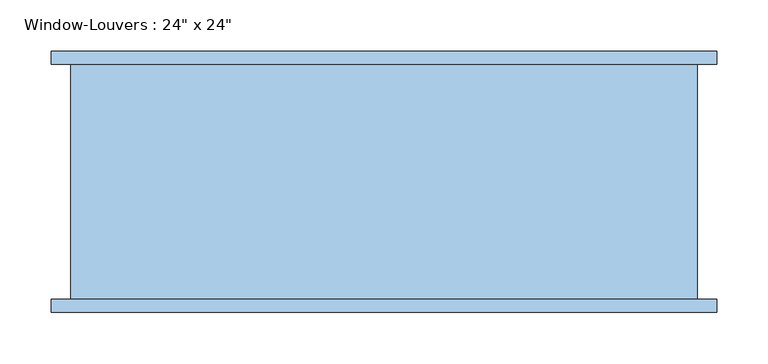
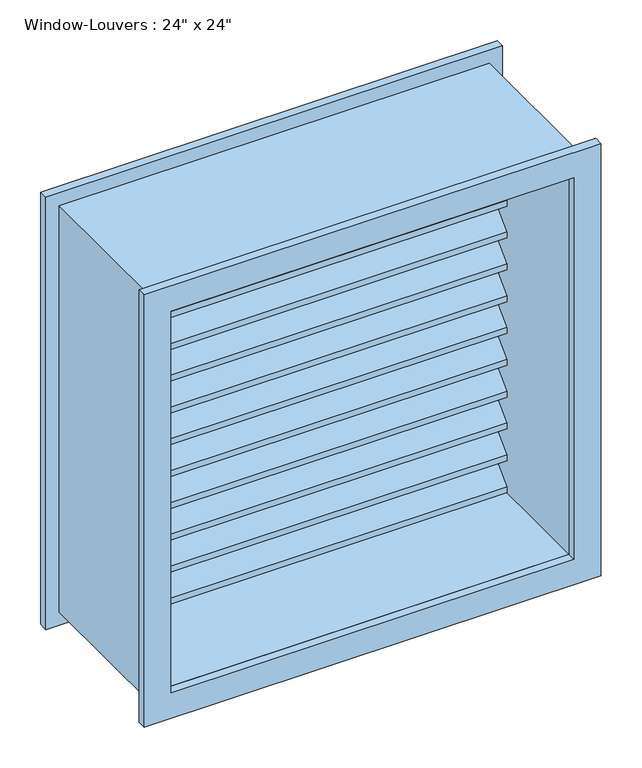
"""IFC4 building model written with IfcOpenShell, lengths in millimetres: window geometry."""

from ifc_helpers import new_model, si_unit, frame, origin, place, context, project, spatial, polyline, outline, extrude, source, transform, mapped, element, save


def window_f2d8fef0(model_context):
    return source(origin(), model_context, "Body", "SweptSolid", [
        extrude(outline(polyline([(107.95, 1419.1754778), (107.95, 1410.1952217), (69.85, 1448.2952217), (31.75, 1410.1952217), (31.75, 1419.1754778), (69.85, 1457.2754778), (107.95, 1419.1754778)])), frame((-285.75, 0.0, 0.0), z_axis=(1.0, 0.0, 0.0), x_axis=(0.0, 1.0, 0.0)), (0.0, 0.0, 1.0), 571.5),
        extrude(outline(polyline([(107.95, 1371.5009557), (107.95, 1362.5206995), (69.85, 1400.6206995), (31.75, 1362.5206995), (31.75, 1371.5009557), (69.85, 1409.6009557), (107.95, 1371.5009557)])), frame((-285.75, 0.0, 0.0), z_axis=(1.0, 0.0, 0.0), x_axis=(0.0, 1.0, 0.0)), (0.0, 0.0, 1.0), 571.5),
        extrude(outline(polyline([(107.95, 1323.8264335), (107.95, 1314.8461774), (69.85, 1352.9461774), (31.75, 1314.8461774), (31.75, 1323.8264335), (69.85, 1361.9264335), (107.95, 1323.8264335)])), frame((-285.75, 0.0, 0.0), z_axis=(1.0, 0.0, 0.0), x_axis=(0.0, 1.0, 0.0)), (0.0, 0.0, 1.0), 571.5),
        extrude(outline(polyline([(107.95, 1276.1519113), (107.95, 1267.1716552), (69.85, 1305.2716552), (31.75, 1267.1716552), (31.75, 1276.1519113), (69.85, 1314.2519113), (107.95, 1276.1519113)])), frame((-285.75, 0.0, 0.0), z_axis=(1.0, 0.0, 0.0), x_axis=(0.0, 1.0, 0.0)), (0.0, 0.0, 1.0), 571.5),
        extrude(outline(polyline([(107.95, 1228.4773891), (107.95, 1219.497133), (69.85, 1257.597133), (31.75, 1219.497133), (31.75, 1228.4773891), (69.85, 1266.5773891), (107.95, 1228.4773891)])), frame((-285.75, 0.0, 0.0), z_axis=(1.0, 0.0, 0.0), x_axis=(0.0, 1.0, 0.0)), (0.0, 0.0, 1.0), 571.5),
        extrude(outline(polyline([(107.95, 1180.802867), (107.95, 1171.8226109), (69.85, 1209.9226109), (31.75, 1171.8226109), (31.75, 1180.802867), (69.85, 1218.902867), (107.95, 1180.802867)])), frame((-285.75, 0.0, 0.0), z_axis=(1.0, 0.0, 0.0), x_axis=(0.0, 1.0, 0.0)), (0.0, 0.0, 1.0), 571.5),
        extrude(outline(polyline([(107.95, 1133.1283448), (107.95, 1124.1480887), (69.85, 1162.2480887), (31.75, 1124.1480887), (31.75, 1133.1283448), (69.85, 1171.2283448), (107.95, 1133.1283448)])), frame((-285.75, 0.0, 0.0), z_axis=(1.0, 0.0, 0.0), x_axis=(0.0, 1.0, 0.0)), (0.0, 0.0, 1.0), 571.5),
        extrude(outline(polyline([(107.95, 1085.4538226), (107.95, 1076.4735665), (69.85, 1114.5735665), (31.75, 1076.4735665), (31.75, 1085.4538226), (69.85, 1123.5538226), (107.95, 1085.4538226)])), frame((-285.75, 0.0, 0.0), z_axis=(1.0, 0.0, 0.0), x_axis=(0.0, 1.0, 0.0)), (0.0, 0.0, 1.0), 571.5),
        extrude(outline(polyline([(107.95, 1037.7793005), (107.95, 1028.7990443), (69.85, 1066.8990443), (31.75, 1028.7990443), (31.75, 1037.7793005), (69.85, 1075.8793005), (107.95, 1037.7793005)])), frame((-285.75, 0.0, 0.0), z_axis=(1.0, 0.0, 0.0), x_axis=(0.0, 1.0, 0.0)), (0.0, 0.0, 1.0), 571.5),
        extrude(outline(polyline([(107.95, 990.1047783), (107.95, 981.1245222), (69.85, 1019.2245222), (31.75, 981.1245222), (31.75, 990.1047783), (69.85, 1028.2047783), (107.95, 990.1047783)])), frame((-285.75, 0.0, 0.0), z_axis=(1.0, 0.0, 0.0), x_axis=(0.0, 1.0, 0.0)), (0.0, 0.0, 1.0), 571.5),
        extrude(outline(polyline([(107.95, 1466.85), (107.95, 1457.8697439), (69.85, 1495.9697439), (31.75, 1457.8697439), (31.75, 1466.85), (69.85, 1504.95), (107.95, 1466.85)])), frame((-285.75, 0.0, 0.0), z_axis=(1.0, 0.0, 0.0), x_axis=(0.0, 1.0, 0.0)), (0.0, 0.0, 1.0), 571.5),
        extrude(outline(polyline([(107.95, 942.4302561), (107.95, 933.45), (69.85, 971.55), (31.75, 933.45), (31.75, 942.4302561), (69.85, 980.5302561), (107.95, 942.4302561)])), frame((-285.75, 0.0, 0.0), z_axis=(1.0, 0.0, 0.0), x_axis=(0.0, 1.0, 0.0)), (0.0, 0.0, 1.0), 571.5),
        extrude(outline(polyline([(1524.0, 304.8), (1524.0, -304.8), (914.4, -304.8), (914.4, 304.8), (1524.0, 304.8)]), holes=[polyline([(1504.95, 285.75), (933.45, 285.75), (933.45, -285.75), (1504.95, -285.75), (1504.95, 285.75)])]), frame((0.0, -120.65, 0.0), z_axis=(0.0, 1.0, 0.0), x_axis=(0.0, 0.0, 1.0)), (0.0, 0.0, 1.0), 228.6),
        extrude(outline(polyline([(1543.05, 323.85), (1543.05, -323.85), (895.35, -323.85), (895.35, 323.85), (1543.05, 323.85)]), holes=[polyline([(1504.95, 285.75), (933.45, 285.75), (933.45, -285.75), (1504.95, -285.75), (1504.95, 285.75)])]), frame((0.0, -133.35, 0.0), z_axis=(0.0, 1.0, 0.0), x_axis=(0.0, 0.0, 1.0)), (0.0, 0.0, 1.0), 12.7),
        extrude(outline(polyline([(1543.05, -323.85), (895.35, -323.85), (895.35, 323.85), (1543.05, 323.85), (1543.05, -323.85)]), holes=[polyline([(1504.95, -285.75), (1504.95, 285.75), (933.45, 285.75), (933.45, -285.75), (1504.95, -285.75)])]), frame((0.0, 107.95, 0.0), z_axis=(0.0, 1.0, 0.0), x_axis=(0.0, 0.0, 1.0)), (0.0, 0.0, 1.0), 12.7),
    ])


if __name__ == "__main__":
    model = new_model("IFC4")
    model_context = context("Model", 3, world=origin())
    ifc_project = project(units=[si_unit("LENGTHUNIT", "METRE", prefix="MILLI")], contexts=[model_context])
    site = spatial("IfcSite", under=ifc_project)
    building = spatial("IfcBuilding", under=site)
    placement = place(None, origin())
    window_shape = window_f2d8fef0(model_context)
    element("IfcWindow", 1, ObjectType="Window-Louvers : 24\" x 24\"", at=placement, inside=building, context=model_context, shape_type="MappedRepresentation", body=[
        mapped(window_shape, transform((0.0, 0.0, 0.0), x_axis=(1.0, 0.0, 0.0), y_axis=(0.0, 1.0, 0.0), z_axis=(0.0, 0.0, 1.0))),
    ])
    save(model, "model.ifc")

# Revit data of these elements
# Type "Window-Louvers : 24\" x 24\""
#   Type Mark = "42"
#   Construction Type Id = "GSP4R"
#   Assembly Code = "B20"
#   Analytic Construction = "1/8 in Pilkington single glazing"
#   Visual Light Transmittance = 0.9
#   Thermal Resistance (R) = 1.53941 (h·ft²·°F)/BTU
#   Solar Heat Gain Coefficient = 0.78
#   Max Height = 1' - 11.74264"
#   Height = 2' - 0"
#   Heat Transfer Coefficient (U) = 0.6496 BTU/(h·ft²·°F)
#   Blade Width [instance default] = 1' - 10 1/2"
#   Blade Vertical Thickness = 0' - 0.35355"
#   Blade Thickness = 0' - 0 1/4"
#   Blade Spacing = 0' - 1 1/2"
#   Blade Height = 0' - 1.85355"
#   Blade Depth = 0' - 3"
#   Blade Angle = 45.00°
#   Default Sill Height = 3' - 0"
#   Trim Projection_Exterior = 0' - 0 1/2"
#   Trim Projection_Interior = 0' - 0 1/2"
#   Trim Width_Exterior = 0' - 1 1/2"
#   Trim Width_Interior = 0' - 1 1/2"
#   Width = 2' - 0"
#   Max Blade Count = 12
#   Define Thermal Properties by = 1
#   Blade Count = 12
#   Frame Material = Birch
#   Louver Material = Birch
#   Trim Exterior Material = Birch
#   Trim Interior Material = Birch
#   Wall Closure = (empty or 0)
# Element 1 (IfcWindow, "Window-Louvers : 24\" x 24\"")
#   Materials on its faces: "Birch"
# Materials
#   "Birch": class "Wood", colour RGB 224 178 126, transparency 0, Description = "Betula Alleghaniensis", Cost = 0
